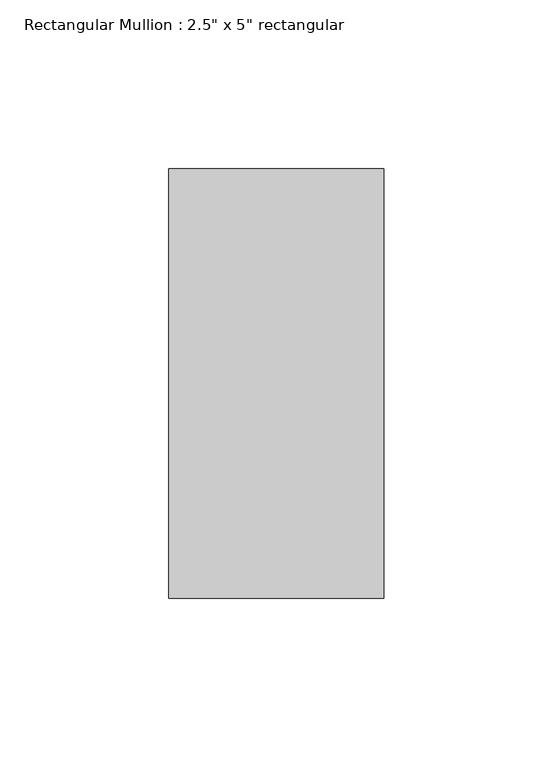
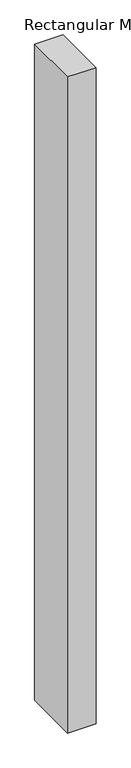
"""IFC4 building model written with IfcOpenShell, lengths in millimetres: member geometry."""

from ifc_helpers import new_model, si_unit, frame, origin, place, context, project, spatial, polyline, outline, extrude, source, transform, mapped, element, save


def member_15f14dc2(model_context):
    return source(origin(), model_context, "Body", "SweptSolid", [
        extrude(outline(polyline([(0.0, 63.5), (0.0, -63.5), (-63.5, -63.5), (-63.5, 63.5), (0.0, 63.5)])), frame((0.0, 0.0, -1547.2824814), z_axis=(0.0, 0.0, 1.0), x_axis=(1.0, 0.0, 0.0)), (0.0, 0.0, 1.0), 1547.2824814),
    ])


if __name__ == "__main__":
    model = new_model("IFC4")
    model_context = context("Model", 3, world=origin())
    ifc_project = project(units=[si_unit("LENGTHUNIT", "METRE", prefix="MILLI")], contexts=[model_context])
    site = spatial("IfcSite", under=ifc_project)
    building = spatial("IfcBuilding", under=site)
    placement = place(None, origin())
    member_shape = member_15f14dc2(model_context)
    element("IfcMember", 1, ObjectType="Rectangular Mullion : 2.5\" x 5\" rectangular", at=placement, inside=building, context=model_context, shape_type="MappedRepresentation", body=[
        mapped(member_shape, transform((0.0, 0.0, 0.0), x_axis=(1.0, 0.0, 0.0), y_axis=(0.0, 1.0, 0.0), z_axis=(0.0, 0.0, 1.0))),
    ])
    save(model, "model.ifc")

# Revit data of these elements
# Type "Rectangular Mullion : 2.5\" x 5\" rectangular"
#   built-in parameter 1007304 = 0.416667 (stored number, unit not read)
#   built-in parameter 1007301 = 0.104167 (stored number, unit not read)
#   built-in parameter 1007300 = 0.104167 (stored number, unit not read)
# Element 1 (IfcMember, "Rectangular Mullion : 2.5\" x 5\" rectangular")
#   Materials on its faces: "Aluminum"
# Materials
#   "Aluminum": class "Metal", colour RGB 247 247 247, transparency 0, Description = "Aluminum 6061", Cost = 0
